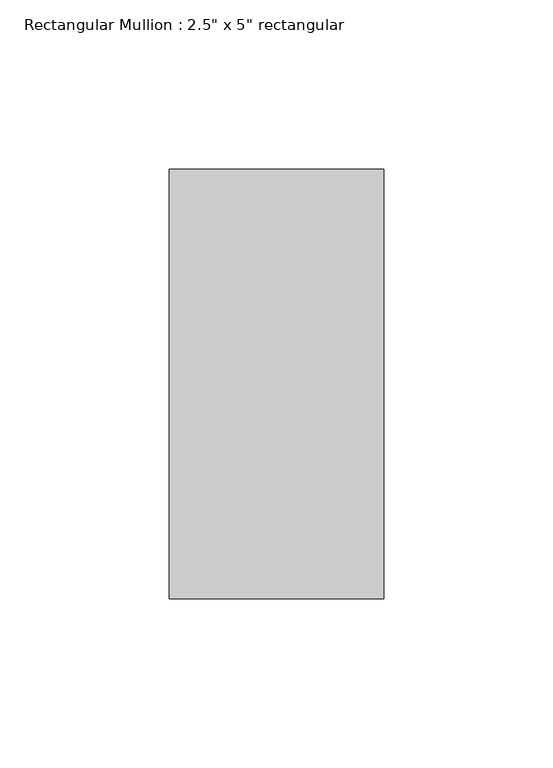
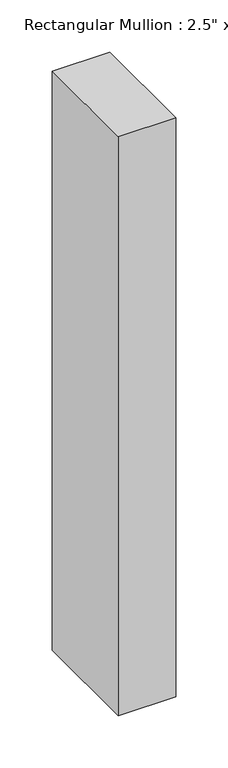
"""IFC4 building model written with IfcOpenShell, lengths in millimetres: member geometry."""

from ifc_helpers import new_model, si_unit, frame, origin, place, context, project, spatial, polyline, outline, extrude, source, transform, mapped, element, save


def member_26d576e8(model_context):
    return source(origin(), model_context, "Body", "SweptSolid", [
        extrude(outline(polyline([(0.0, 63.5), (0.0, -63.5), (-63.5, -63.5), (-63.5, 63.5), (0.0, 63.5)])), frame((0.0, 0.0, -677.3333333), z_axis=(0.0, 0.0, 1.0), x_axis=(1.0, 0.0, 0.0)), (0.0, 0.0, 1.0), 677.3333333),
    ])


if __name__ == "__main__":
    model = new_model("IFC4")
    model_context = context("Model", 3, world=origin())
    ifc_project = project(units=[si_unit("LENGTHUNIT", "METRE", prefix="MILLI")], contexts=[model_context])
    site = spatial("IfcSite", under=ifc_project)
    building = spatial("IfcBuilding", under=site)
    placement = place(None, origin())
    member_shape = member_26d576e8(model_context)
    element("IfcMember", 1, ObjectType="Rectangular Mullion : 2.5\" x 5\" rectangular", at=placement, inside=building, context=model_context, shape_type="MappedRepresentation", body=[
        mapped(member_shape, transform((0.0, 0.0, 0.0), x_axis=(1.0, 0.0, 0.0), y_axis=(0.0, 1.0, 0.0), z_axis=(0.0, 0.0, 1.0))),
    ])
    save(model, "model.ifc")

# Revit data of these elements
# Type "Rectangular Mullion : 2.5\" x 5\" rectangular"
#   built-in parameter 1007304 = 0.416667 (stored number, unit not read)
#   built-in parameter 1007301 = 0.104167 (stored number, unit not read)
#   built-in parameter 1007300 = 0.104167 (stored number, unit not read)
# Element 1 (IfcMember, "Rectangular Mullion : 2.5\" x 5\" rectangular")
#   Materials on its faces: "Aluminum"
# Materials
#   "Aluminum": class "Metal", colour RGB 247 247 247, transparency 0, Description = "Aluminum 6061", Cost = 0
